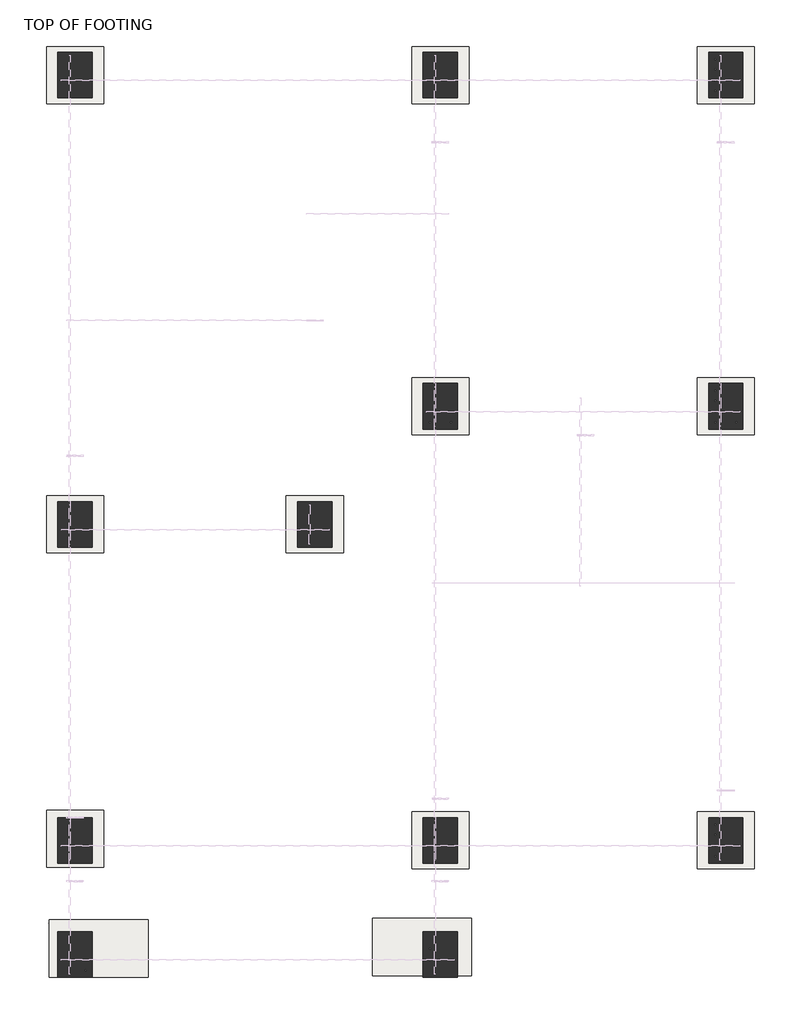
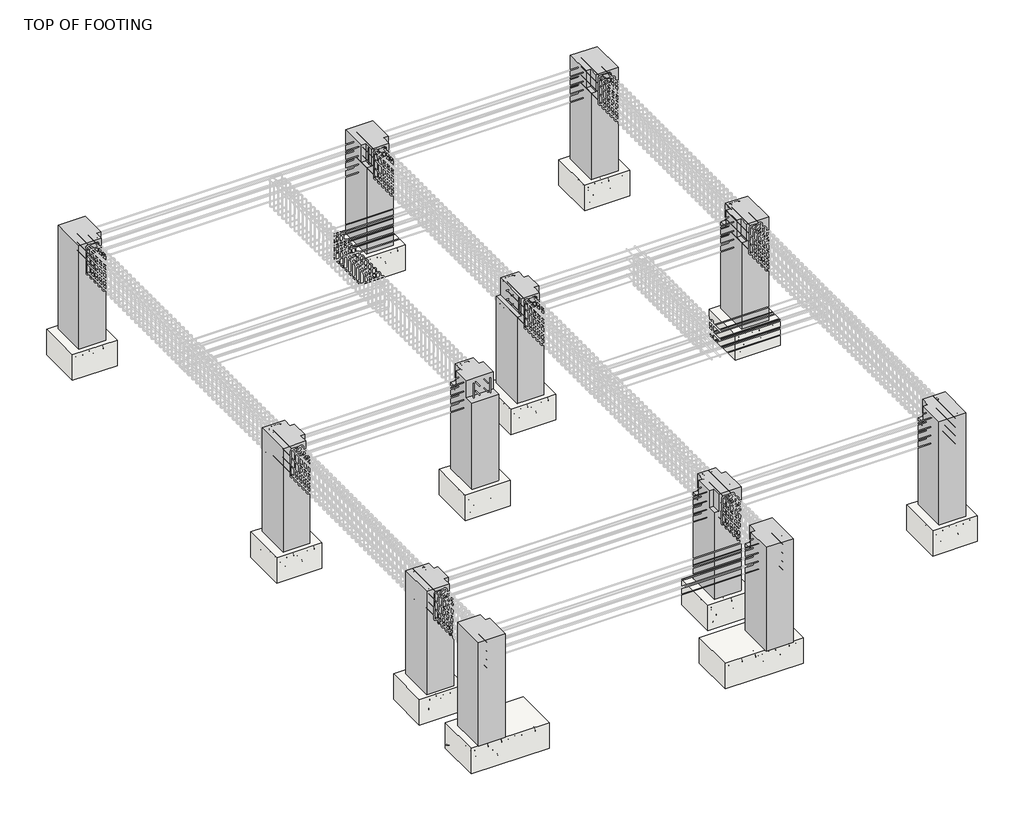
# One storey, part 1 of 8: 12 columns, 12 slabs.
"""IFC4 building model written with IfcOpenShell, lengths in millimetres."""

from ifc_helpers import new_model, si_unit, origin, place, context, project, spatial, faceted_brep, transform, mapped, element, save
from components import m_footing_rectangular_1300mm_x_750mm_x_450mm_70b2c142, m_footing_rectangular_750mm_x_750mm_x_450mm_d1bf6791

model = new_model("IFC4")

# Units and contexts
model_context = context("Model", 3, world=origin())
ifc_project = project(units=[si_unit("LENGTHUNIT", "METRE", prefix="MILLI")], contexts=[model_context])

# Site, building, storey
site = spatial("IfcSite", under=ifc_project)
building = spatial("IfcBuilding", under=site)
storey = spatial("IfcBuildingStorey", under=building, Name="TOP OF FOOTING", Elevation=-1828.8)

# Columns
placement = place(None, origin())
element("IfcColumn", 1, ObjectType="M_Concrete-Rectangular-Column : 450 x 600mm", at=placement, inside=storey, context=model_context, shape_type="Brep", body=[
    faceted_brep([(-6277.4961367, 9866.9920243, -1828.8), (-6277.4961367, 9266.9920243, -1828.8), (-6727.4961367, 9266.9920243, -1828.8), (-6727.4961367, 9866.9920243, -1828.8), (-6277.4961367, 9866.9920243, 0.0), (-6277.4961367, 9416.9920243, 0.0), (-6277.4961367, 9416.9920243, -300.0), (-6277.4961367, 9266.9920243, -300.0), (-6352.4961367, 9266.9920243, -300.0), (-6352.4961367, 9266.9920243, 0.0), (-6727.4961367, 9266.9920243, 0.0), (-6727.4961367, 9866.9920243, 0.0), (-6352.4961367, 9416.9920243, 0.0), (-6352.4961367, 9416.9920243, -300.0)], [[[0, 1, 2, 3]], [[1, 0, 4, 5, 6, 7]], [[2, 1, 7, 8, 9, 10]], [[3, 2, 10, 11]], [[0, 3, 11, 4]], [[11, 10, 9, 12, 5, 4]], [[13, 8, 7, 6]], [[12, 13, 6, 5]], [[13, 12, 9, 8]]]),
])
element("IfcColumn", 2, ObjectType="M_Concrete-Rectangular-Column : 450 x 600mm", at=placement, inside=storey, context=model_context, shape_type="Brep", body=[
    faceted_brep([(2272.5038633, 9866.9920243, -1828.8), (2272.5038633, 9266.9920243, -1828.8), (1822.5038633, 9266.9920243, -1828.8), (1822.5038633, 9866.9920243, -1828.8), (2272.5038633, 9866.9920243, 0.0), (2272.5038633, 9266.9920243, 0.0), (1897.5038633, 9266.9920243, 0.0), (1897.5038633, 9266.9920243, -300.0), (1822.5038633, 9266.9920243, -300.0), (1822.5038633, 9416.9920243, -300.0), (1822.5038633, 9416.9920243, 0.0), (1822.5038633, 9866.9920243, 0.0), (1897.5038633, 9416.9920243, 0.0), (1897.5038633, 9416.9920243, -300.0)], [[[0, 1, 2, 3]], [[1, 0, 4, 5]], [[2, 1, 5, 6, 7, 8]], [[3, 2, 8, 9, 10, 11]], [[0, 3, 11, 4]], [[5, 4, 11, 10, 12, 6]], [[7, 13, 9, 8]], [[13, 12, 10, 9]], [[12, 13, 7, 6]]]),
])
element("IfcColumn", 3, ObjectType="M_Concrete-Rectangular-Column : 450 x 600mm", at=placement, inside=storey, context=model_context, shape_type="Brep", body=[
    faceted_brep([(-6277.4961367, -1683.0079757, -1828.8), (-6277.4961367, -2283.0079757, -1828.8), (-6727.4961367, -2283.0079757, -1828.8), (-6727.4961367, -1683.0079757, -1828.8), (-6277.4961367, -1683.0079757, -300.0), (-6277.4961367, -1833.0079757, -300.0), (-6277.4961367, -1833.0079757, 0.0), (-6277.4961367, -2283.0079757, 0.0), (-6727.4961367, -2283.0079757, 0.0), (-6727.4961367, -1683.0079757, 0.0), (-6352.4961367, -1683.0079757, 0.0), (-6352.4961367, -1683.0079757, -300.0), (-6352.4961367, -1833.0079757, 0.0), (-6352.4961367, -1833.0079757, -300.0)], [[[0, 1, 2, 3]], [[1, 0, 4, 5, 6, 7]], [[2, 1, 7, 8]], [[3, 2, 8, 9]], [[0, 3, 9, 10, 11, 4]], [[8, 7, 6, 12, 10, 9]], [[13, 5, 4, 11]], [[12, 13, 11, 10]], [[13, 12, 6, 5]]]),
])
element("IfcColumn", 4, ObjectType="M_Concrete-Rectangular-Column : 450 x 600mm", at=placement, inside=storey, context=model_context, shape_type="Brep", body=[
    faceted_brep([(-1477.4961367, 9866.9920243, -1828.8), (-1477.4961367, 9266.9920243, -1828.8), (-1927.4961367, 9266.9920243, -1828.8), (-1927.4961367, 9866.9920243, -1828.8), (-1477.4961367, 9866.9920243, 0.0), (-1477.4961367, 9416.9920243, 0.0), (-1477.4961367, 9416.9920243, -300.0), (-1477.4961367, 9266.9920243, -300.0), (-1552.4961367, 9266.9920243, -300.0), (-1552.4961367, 9266.9920243, 0.0), (-1852.4961367, 9266.9920243, 0.0), (-1852.4961367, 9266.9920243, -300.0), (-1927.4961367, 9266.9920243, -300.0), (-1927.4961367, 9416.9920243, -300.0), (-1927.4961367, 9416.9920243, 0.0), (-1927.4961367, 9866.9920243, 0.0), (-1852.4961367, 9416.9920243, 0.0), (-1552.4961367, 9416.9920243, 0.0), (-1552.4961367, 9416.9920243, -300.0), (-1852.4961367, 9416.9920243, -300.0)], [[[0, 1, 2, 3]], [[1, 0, 4, 5, 6, 7]], [[2, 1, 7, 8, 9, 10, 11, 12]], [[3, 2, 12, 13, 14, 15]], [[0, 3, 15, 4]], [[4, 15, 14, 16, 10, 9, 17, 5]], [[18, 8, 7, 6]], [[17, 18, 6, 5]], [[18, 17, 9, 8]], [[19, 16, 14, 13]], [[16, 19, 11, 10]], [[11, 19, 13, 12]]]),
])
element("IfcColumn", 5, ObjectType="M_Concrete-Rectangular-Column : 450 x 600mm", at=placement, inside=storey, context=model_context, shape_type="Brep", body=[
    faceted_brep([(2272.5038633, 5516.9920243, -1828.8), (2272.5038633, 4916.9920243, -1828.8), (1822.5038633, 4916.9920243, -1828.8), (1822.5038633, 5516.9920243, -1828.8), (2272.5038633, 5516.9920243, 0.0), (2272.5038633, 4916.9920243, 0.0), (1897.5038633, 4916.9920243, 0.0), (1897.5038633, 4916.9920243, -300.0), (1822.5038633, 4916.9920243, -300.0), (1822.5038633, 5066.9920243, -300.0), (1822.5038633, 5066.9920243, 0.0), (1822.5038633, 5366.9920243, 0.0), (1822.5038633, 5366.9920243, -300.0), (1822.5038633, 5516.9920243, -300.0), (1897.5038633, 5516.9920243, -300.0), (1897.5038633, 5516.9920243, 0.0), (1897.5038633, 5366.9920243, 0.0), (1897.5038633, 5066.9920243, 0.0), (1897.5038633, 5366.9920243, -300.0), (1897.5038633, 5066.9920243, -300.0)], [[[0, 1, 2, 3]], [[1, 0, 4, 5]], [[2, 1, 5, 6, 7, 8]], [[3, 2, 8, 9, 10, 11, 12, 13]], [[0, 3, 13, 14, 15, 4]], [[5, 4, 15, 16, 11, 10, 17, 6]], [[12, 18, 14, 13]], [[18, 16, 15, 14]], [[16, 18, 12, 11]], [[19, 9, 8, 7]], [[9, 19, 17, 10]], [[17, 19, 7, 6]]]),
])
element("IfcColumn", 6, ObjectType="M_Concrete-Rectangular-Column : 450 x 600mm", at=placement, inside=storey, context=model_context, shape_type="Brep", body=[
    faceted_brep([(-1477.4961367, 5516.9920243, -1828.8), (-1477.4961367, 4916.9920243, -1828.8), (-1927.4961367, 4916.9920243, -1828.8), (-1927.4961367, 5516.9920243, -1828.8), (-1477.4961367, 5516.9920243, -300.0), (-1477.4961367, 5366.9920243, -300.0), (-1477.4961367, 5366.9920243, 0.0), (-1477.4961367, 5066.9920243, 0.0), (-1477.4961367, 5066.9920243, -300.0), (-1477.4961367, 4916.9920243, -300.0), (-1552.4961367, 4916.9920243, -300.0), (-1552.4961367, 4916.9920243, 0.0), (-1852.4961367, 4916.9920243, 0.0), (-1852.4961367, 4916.9920243, -300.0), (-1927.4961367, 4916.9920243, -300.0), (-1927.4961367, 5516.9920243, -300.0), (-1852.4961367, 5516.9920243, -300.0), (-1852.4961367, 5516.9920243, 0.0), (-1552.4961367, 5516.9920243, 0.0), (-1552.4961367, 5516.9920243, -300.0), (-1552.4961367, 5366.9920243, 0.0), (-1552.4961367, 5066.9920243, 0.0), (-1552.4961367, 5366.9920243, -300.0), (-1552.4961367, 5066.9920243, -300.0)], [[[0, 1, 2, 3]], [[1, 0, 4, 5, 6, 7, 8, 9]], [[2, 1, 9, 10, 11, 12, 13, 14]], [[3, 2, 14, 15]], [[0, 3, 15, 16, 17, 18, 19, 4]], [[6, 20, 18, 17, 12, 11, 21, 7]], [[19, 22, 5, 4]], [[22, 20, 6, 5]], [[20, 22, 19, 18]], [[16, 13, 12, 17]], [[13, 16, 15, 14]], [[8, 23, 10, 9]], [[23, 21, 11, 10]], [[23, 8, 7, 21]]]),
])
element("IfcColumn", 7, ObjectType="M_Concrete-Rectangular-Column : 450 x 600mm", at=placement, inside=storey, context=model_context, shape_type="Brep", body=[
    faceted_brep([(-6277.4961367, 3966.9920243, -1828.8), (-6277.4961367, 3366.9920243, -1828.8), (-6727.4961367, 3366.9920243, -1828.8), (-6727.4961367, 3966.9920243, -1828.8), (-6277.4961367, 3966.9920243, -300.0), (-6277.4961367, 3816.9920243, -300.0), (-6277.4961367, 3816.9920243, 0.0), (-6277.4961367, 3521.9920243, 0.0), (-6277.4961367, 3521.9920243, -300.0), (-6277.4961367, 3366.9920243, -300.0), (-6347.4961367, 3366.9920243, -300.0), (-6347.4961367, 3366.9920243, 0.0), (-6727.4961367, 3366.9920243, 0.0), (-6727.4961367, 3966.9920243, 0.0), (-6352.4961367, 3966.9920243, 0.0), (-6352.4961367, 3966.9920243, -300.0), (-6347.4961367, 3521.9920243, 0.0), (-6352.4961367, 3816.9920243, 0.0), (-6347.4961367, 3521.9920243, -300.0), (-6352.4961367, 3816.9920243, -300.0)], [[[0, 1, 2, 3]], [[1, 0, 4, 5, 6, 7, 8, 9]], [[2, 1, 9, 10, 11, 12]], [[3, 2, 12, 13]], [[0, 3, 13, 14, 15, 4]], [[13, 12, 11, 16, 7, 6, 17, 14]], [[18, 10, 9, 8]], [[16, 18, 8, 7]], [[18, 16, 11, 10]], [[5, 19, 17, 6]], [[17, 19, 15, 14]], [[19, 5, 4, 15]]]),
])
element("IfcColumn", 8, ObjectType="M_Concrete-Rectangular-Column : 450 x 600mm", at=placement, inside=storey, context=model_context, shape_type="Brep", body=[
    faceted_brep([(-3127.4961367, 3966.9920243, -1828.8), (-3127.4961367, 3366.9920243, -1828.8), (-3577.4961367, 3366.9920243, -1828.8), (-3577.4961367, 3966.9920243, -1828.8), (-3127.4961367, 3966.9920243, -300.0), (-3127.4961367, 3816.9920243, -300.0), (-3127.4961367, 3816.9920243, 0.0), (-3127.4961367, 3521.9920243, 0.0), (-3127.4961367, 3521.9920243, -300.0), (-3127.4961367, 3366.9920243, -300.0), (-3577.4961367, 3366.9920243, -300.0), (-3577.4961367, 3521.9920243, -300.0), (-3577.4961367, 3521.9920243, 0.0), (-3577.4961367, 3816.9920243, 0.0), (-3577.4961367, 3816.9920243, -300.0), (-3577.4961367, 3966.9920243, -300.0), (-3502.4961367, 3966.9920243, -300.0), (-3502.4961367, 3966.9920243, 0.0), (-3202.4961367, 3966.9920243, 0.0), (-3202.4961367, 3966.9920243, -300.0), (-3202.4961367, 3816.9920243, 0.0), (-3502.4961367, 3816.9920243, 0.0), (-3502.4961367, 3816.9920243, -300.0), (-3202.4961367, 3816.9920243, -300.0)], [[[0, 1, 2, 3]], [[1, 0, 4, 5, 6, 7, 8, 9]], [[2, 1, 9, 10]], [[3, 2, 10, 11, 12, 13, 14, 15]], [[0, 3, 15, 16, 17, 18, 19, 4]], [[12, 7, 6, 20, 18, 17, 21, 13]], [[8, 11, 10, 9]], [[11, 8, 7, 12]], [[22, 21, 17, 16]], [[21, 22, 14, 13]], [[23, 20, 6, 5]], [[20, 23, 19, 18]], [[19, 23, 5, 4]], [[14, 22, 16, 15]]]),
])
element("IfcColumn", 9, ObjectType="M_Concrete-Rectangular-Column : 450 x 600mm", at=placement, inside=storey, context=model_context, shape_type="Brep", body=[
    faceted_brep([(-6277.4961367, -183.0079757, -1828.8), (-6277.4961367, -783.0079757, -1828.8), (-6727.4961367, -783.0079757, -1828.8), (-6727.4961367, -183.0079757, -1828.8), (-6277.4961367, -183.0079757, -300.0), (-6277.4961367, -333.0079757, -300.0), (-6277.4961367, -333.0079757, 0.0), (-6277.4961367, -633.0079757, 0.0), (-6277.4961367, -633.0079757, -300.0), (-6277.4961367, -783.0079757, -300.0), (-6352.4961367, -783.0079757, -300.0), (-6352.4961367, -783.0079757, 0.0), (-6727.4961367, -783.0079757, 0.0), (-6727.4961367, -183.0079757, 0.0), (-6347.4961367, -183.0079757, 0.0), (-6347.4961367, -183.0079757, -300.0), (-6352.4961367, -633.0079757, 0.0), (-6347.4961367, -333.0079757, 0.0), (-6347.4961367, -333.0079757, -300.0), (-6352.4961367, -633.0079757, -300.0)], [[[0, 1, 2, 3]], [[1, 0, 4, 5, 6, 7, 8, 9]], [[2, 1, 9, 10, 11, 12]], [[3, 2, 12, 13]], [[0, 3, 13, 14, 15, 4]], [[13, 12, 11, 16, 7, 6, 17, 14]], [[15, 18, 5, 4]], [[18, 17, 6, 5]], [[17, 18, 15, 14]], [[8, 19, 10, 9]], [[19, 16, 11, 10]], [[16, 19, 8, 7]]]),
])
element("IfcColumn", 10, ObjectType="M_Concrete-Rectangular-Column : 450 x 600mm", at=placement, inside=storey, context=model_context, shape_type="Brep", body=[
    faceted_brep([(-1477.4961367, -183.0079757, -1828.8), (-1477.4961367, -783.0079757, -1828.8), (-1927.4961367, -783.0079757, -1828.8), (-1927.4961367, -183.0079757, -1828.8), (-1477.4961367, -183.0079757, -300.0), (-1477.4961367, -333.0079757, -300.0), (-1477.4961367, -333.0079757, 0.0), (-1477.4961367, -783.0079757, 0.0), (-1852.4961367, -783.0079757, 0.0), (-1852.4961367, -783.0079757, -300.0), (-1927.4961367, -783.0079757, -300.0), (-1927.4961367, -633.0079757, -300.0), (-1927.4961367, -633.0079757, 0.0), (-1927.4961367, -333.0079757, 0.0), (-1927.4961367, -333.0079757, -300.0), (-1927.4961367, -183.0079757, -300.0), (-1857.4961367, -183.0079757, -300.0), (-1857.4961367, -183.0079757, 0.0), (-1552.4961367, -183.0079757, 0.0), (-1552.4961367, -183.0079757, -300.0), (-1552.4961367, -333.0079757, 0.0), (-1857.4961367, -333.0079757, 0.0), (-1852.4961367, -633.0079757, 0.0), (-1552.4961367, -333.0079757, -300.0), (-1857.4961367, -333.0079757, -300.0), (-1852.4961367, -633.0079757, -300.0)], [[[0, 1, 2, 3]], [[1, 0, 4, 5, 6, 7]], [[2, 1, 7, 8, 9, 10]], [[3, 2, 10, 11, 12, 13, 14, 15]], [[0, 3, 15, 16, 17, 18, 19, 4]], [[7, 6, 20, 18, 17, 21, 13, 12, 22, 8]], [[19, 23, 5, 4]], [[23, 20, 6, 5]], [[20, 23, 19, 18]], [[14, 24, 16, 15]], [[24, 21, 17, 16]], [[21, 24, 14, 13]], [[9, 25, 11, 10]], [[25, 22, 12, 11]], [[22, 25, 9, 8]]]),
])
element("IfcColumn", 11, ObjectType="M_Concrete-Rectangular-Column : 450 x 600mm", at=placement, inside=storey, context=model_context, shape_type="Brep", body=[
    faceted_brep([(2272.5038633, -183.0079757, -1828.8), (2272.5038633, -783.0079757, -1828.8), (1822.5038633, -783.0079757, -1828.8), (1822.5038633, -183.0079757, -1828.8), (2272.5038633, -183.0079757, 0.0), (2272.5038633, -783.0079757, 0.0), (1822.5038633, -783.0079757, 0.0), (1822.5038633, -333.0079757, 0.0), (1822.5038633, -333.0079757, -300.0), (1822.5038633, -183.0079757, -300.0), (1897.5038633, -183.0079757, -300.0), (1897.5038633, -183.0079757, 0.0), (1897.5038633, -333.0079757, 0.0), (1897.5038633, -333.0079757, -300.0)], [[[0, 1, 2, 3]], [[1, 0, 4, 5]], [[2, 1, 5, 6]], [[3, 2, 6, 7, 8, 9]], [[0, 3, 9, 10, 11, 4]], [[5, 4, 11, 12, 7, 6]], [[8, 13, 10, 9]], [[13, 12, 11, 10]], [[12, 13, 8, 7]]]),
])
element("IfcColumn", 12, ObjectType="M_Concrete-Rectangular-Column : 450 x 600mm", at=placement, inside=storey, context=model_context, shape_type="Brep", body=[
    faceted_brep([(-1477.4961367, -1683.0079757, -1828.8), (-1477.4961367, -2283.0079757, -1828.8), (-1927.4961367, -2283.0079757, -1828.8), (-1927.4961367, -1683.0079757, -1828.8), (-1477.4961367, -1683.0079757, 0.0), (-1477.4961367, -2283.0079757, 0.0), (-1927.4961367, -2283.0079757, 0.0), (-1927.4961367, -1833.0079757, 0.0), (-1927.4961367, -1833.0079757, -300.0), (-1927.4961367, -1683.0079757, -300.0), (-1852.4961367, -1683.0079757, -300.0), (-1852.4961367, -1683.0079757, 0.0), (-1852.4961367, -1833.0079757, 0.0), (-1852.4961367, -1833.0079757, -300.0)], [[[0, 1, 2, 3]], [[1, 0, 4, 5]], [[2, 1, 5, 6]], [[3, 2, 6, 7, 8, 9]], [[0, 3, 9, 10, 11, 4]], [[5, 4, 11, 12, 7, 6]], [[8, 13, 10, 9]], [[13, 12, 11, 10]], [[12, 13, 8, 7]]]),
])

# Slabs
m_footing_rectangular_1300mm_x_750mm_x_450mm_shape = m_footing_rectangular_1300mm_x_750mm_x_450mm_70b2c142(model_context)
element("IfcSlab", 13, ObjectType="M_Footing-Rectangular : 1300MM X 750MM X 450MM", at=placement, inside=storey, context=model_context, shape_type="MappedRepresentation", body=[
    mapped(m_footing_rectangular_1300mm_x_750mm_x_450mm_shape, transform((-6192.4961367, -1903.0079757, -1828.8), x_axis=(1.0, 0.0, 0.0), y_axis=(0.0, 1.0, 0.0), z_axis=(0.0, 0.0, 1.0))),
])
element("IfcSlab", 14, ObjectType="M_Footing-Rectangular : 1300MM X 750MM X 450MM", at=placement, inside=storey, context=model_context, shape_type="MappedRepresentation", body=[
    mapped(m_footing_rectangular_1300mm_x_750mm_x_450mm_shape, transform((-1942.4961367, -1883.0079757, -1828.8), x_axis=(1.0, 0.0, 0.0), y_axis=(0.0, 1.0, 0.0), z_axis=(0.0, 0.0, 1.0))),
])
m_footing_rectangular_750mm_x_750mm_x_450mm_shape = m_footing_rectangular_750mm_x_750mm_x_450mm_d1bf6791(model_context)
element("IfcSlab", 15, ObjectType="M_Footing-Rectangular : 750MM X 750MM X 450MM", at=placement, inside=storey, context=model_context, shape_type="MappedRepresentation", body=[
    mapped(m_footing_rectangular_750mm_x_750mm_x_450mm_shape, transform((-6502.4961367, 9566.9920243, -1828.8), x_axis=(1.0, 0.0, 0.0), y_axis=(0.0, 1.0, 0.0), z_axis=(0.0, 0.0, 1.0))),
])
element("IfcSlab", 16, ObjectType="M_Footing-Rectangular : 750MM X 750MM X 450MM", at=placement, inside=storey, context=model_context, shape_type="MappedRepresentation", body=[
    mapped(m_footing_rectangular_750mm_x_750mm_x_450mm_shape, transform((-1702.4961367, 9566.9920243, -1828.8), x_axis=(1.0, 0.0, 0.0), y_axis=(0.0, 1.0, 0.0), z_axis=(0.0, 0.0, 1.0))),
])
element("IfcSlab", 17, ObjectType="M_Footing-Rectangular : 750MM X 750MM X 450MM", at=placement, inside=storey, context=model_context, shape_type="MappedRepresentation", body=[
    mapped(m_footing_rectangular_750mm_x_750mm_x_450mm_shape, transform((2047.5038633, 9566.9920243, -1828.8), x_axis=(1.0, 0.0, 0.0), y_axis=(0.0, 1.0, 0.0), z_axis=(0.0, 0.0, 1.0))),
])
element("IfcSlab", 18, ObjectType="M_Footing-Rectangular : 750MM X 750MM X 450MM", at=placement, inside=storey, context=model_context, shape_type="MappedRepresentation", body=[
    mapped(m_footing_rectangular_750mm_x_750mm_x_450mm_shape, transform((2047.5038633, 5216.9920243, -1828.8), x_axis=(1.0, 0.0, 0.0), y_axis=(0.0, 1.0, 0.0), z_axis=(0.0, 0.0, 1.0))),
])
element("IfcSlab", 19, ObjectType="M_Footing-Rectangular : 750MM X 750MM X 450MM", at=placement, inside=storey, context=model_context, shape_type="MappedRepresentation", body=[
    mapped(m_footing_rectangular_750mm_x_750mm_x_450mm_shape, transform((-1702.4961367, 5216.9920243, -1828.8), x_axis=(1.0, 0.0, 0.0), y_axis=(0.0, 1.0, 0.0), z_axis=(0.0, 0.0, 1.0))),
])
element("IfcSlab", 20, ObjectType="M_Footing-Rectangular : 750MM X 750MM X 450MM", at=placement, inside=storey, context=model_context, shape_type="MappedRepresentation", body=[
    mapped(m_footing_rectangular_750mm_x_750mm_x_450mm_shape, transform((-3352.4961367, 3666.9920243, -1828.8), x_axis=(1.0, 0.0, 0.0), y_axis=(0.0, 1.0, 0.0), z_axis=(0.0, 0.0, 1.0))),
])
element("IfcSlab", 21, ObjectType="M_Footing-Rectangular : 750MM X 750MM X 450MM", at=placement, inside=storey, context=model_context, shape_type="MappedRepresentation", body=[
    mapped(m_footing_rectangular_750mm_x_750mm_x_450mm_shape, transform((-6502.4961367, 3666.9920243, -1828.8), x_axis=(1.0, 0.0, 0.0), y_axis=(0.0, 1.0, 0.0), z_axis=(0.0, 0.0, 1.0))),
])
element("IfcSlab", 22, ObjectType="M_Footing-Rectangular : 750MM X 750MM X 450MM", at=placement, inside=storey, context=model_context, shape_type="MappedRepresentation", body=[
    mapped(m_footing_rectangular_750mm_x_750mm_x_450mm_shape, transform((2047.5038633, -483.0079757, -1828.8), x_axis=(1.0, 0.0, 0.0), y_axis=(0.0, 1.0, 0.0), z_axis=(0.0, 0.0, 1.0))),
])
element("IfcSlab", 23, ObjectType="M_Footing-Rectangular : 750MM X 750MM X 450MM", at=placement, inside=storey, context=model_context, shape_type="MappedRepresentation", body=[
    mapped(m_footing_rectangular_750mm_x_750mm_x_450mm_shape, transform((-1702.4961367, -483.0079757, -1828.8), x_axis=(1.0, 0.0, 0.0), y_axis=(0.0, 1.0, 0.0), z_axis=(0.0, 0.0, 1.0))),
])
element("IfcSlab", 24, ObjectType="M_Footing-Rectangular : 750MM X 750MM X 450MM", at=placement, inside=storey, context=model_context, shape_type="MappedRepresentation", body=[
    mapped(m_footing_rectangular_750mm_x_750mm_x_450mm_shape, transform((-6502.4961367, -463.0079757, -1828.8), x_axis=(1.0, 0.0, 0.0), y_axis=(0.0, 1.0, 0.0), z_axis=(0.0, 0.0, 1.0))),
])

save(model, "model.ifc")

# Revit data of these elements
# Grids (mm)
#   "1": line (-6502.496, -9763.109) -> (-6502.496, 12272.341)
#   "2": line (-3352.496, -9763.109) -> (-3352.496, 12272.341)
#   "3": line (-1702.496, -9763.109) -> (-1702.496, 12272.341)
#   "4": line (2047.504, -9763.109) -> (2047.504, 12272.341)
#   "A": line (-9778.694, 9566.992) -> (3614.786, 9566.992)
#   "B": line (-9778.694, 6416.992) -> (3614.786, 6416.992)
#   "C": line (-9778.694, 5216.992) -> (3614.786, 5216.992)
#   "D": line (-9778.694, 3666.992) -> (3614.786, 3666.992)
#   "E": line (-9778.694, 2966.992) -> (3614.786, 2966.992)
#   "F": line (-9778.694, -483.008) -> (3614.786, -483.008)
#   "G": line (-9778.694, -1983.008) -> (3614.786, -1983.008)
# Type "M_Concrete-Rectangular-Column : 450 x 600mm"
#   b = 450 mm
#   h = 600 mm
#   Structural Material [instance default] = Concrete, Cast-in-Place gray
# Type "M_Footing-Rectangular : 1300MM X 750MM X 450MM"
#   Width = 1300 mm
#   Length = 750 mm
#   Foundation Thickness = 450 mm
#   Structural Material [instance default] = Concrete, Cast-in-Place gray
#   Assembly Code = ""
# Type "M_Footing-Rectangular : 750MM X 750MM X 450MM"
#   Width = 750 mm
#   Length = 750 mm
#   Foundation Thickness = 450 mm
#   Structural Material [instance default] = Concrete, Cast-in-Place gray
#   Assembly Code = ""
# Elements 1, 2, 3, 4, 5, 6, 7, 8, 9, 10, 11, 12 (IfcColumn, "M_Concrete-Rectangular-Column : 450 x 600mm")
#   Structural Material = Concrete, Cast-in-Place gray
#   Phase Created = New Construction
#   Materials on its faces: "Concrete, Cast-in-Place gray"
# Elements 13, 14 (IfcSlab, "M_Footing-Rectangular : 1300MM X 750MM X 450MM")
#   Structural Material = Concrete, Cast-in-Place gray
#   Phase Created = New Construction
#   Materials on its faces: "Concrete, Cast-in-Place gray"
# Elements 15, 16, 17, 18, 19, 20, 21, 22, 23, 24 (IfcSlab, "M_Footing-Rectangular : 750MM X 750MM X 450MM")
#   Structural Material = Concrete, Cast-in-Place gray
#   Phase Created = New Construction
#   Materials on its faces: "Concrete, Cast-in-Place gray"
# Materials
#   "Concrete, Cast-in-Place gray": class "Concrete", colour RGB 192 192 192, transparency 0, Description = "Cast-in-place concrete", Cost = 0
